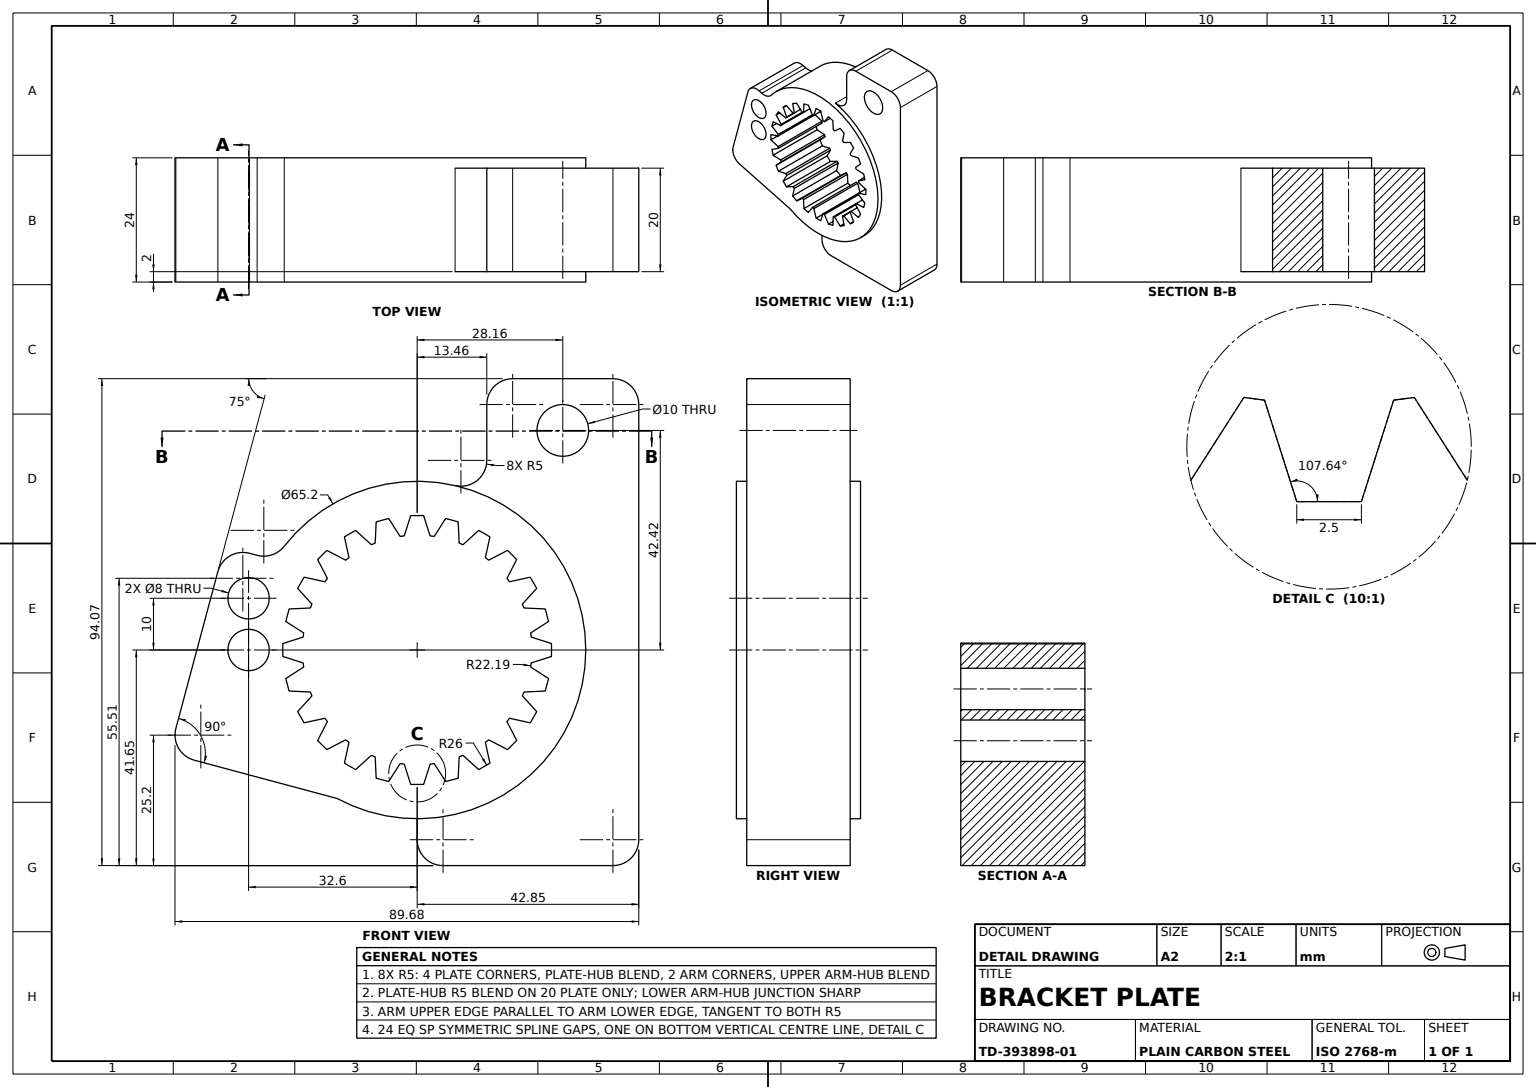
SolidWorks part; units mm, degrees
material "Plain Carbon Steel"
ref_plane "Front Plane" through (0, 0, 0) normal (0, 0, 1) x (1, 0, 0)
ref_plane "Top Plane" through (0, 0, 0) normal (0, 1, 0) x (1, 0, 0)
ref_plane "Right Plane" through (0, 0, 0) normal (1, 0, 0) x (0, 0, -1)
sketch "Splined Hub Profile" plane through (0, 0, 0) normal (0, 0, 1) x (1, 0, 0)
  line L0 (0, 0) -> (0, 32.6) construction
  line L1 (0, 0) -> (0, -32.6) construction
  line L2 (0, 0) -> (32.6, 0) construction
  line L3 (0, 0) -> (-32.6, 0) construction
  line L4 (26, 0) -> (25.97, 1.2496)
  line L5 (26, 0) -> (25.97, -1.2496)
  line L8 (22.0492, 2.496) -> (25.97, 1.2496)
  line L9 (22.0492, -2.496) -> (25.97, -1.2496)
  line L10 (21.9439, -3.2958) -> (25.4085, -5.5145)
  line L11 (20.6518, -8.1177) -> (24.7616, -7.9286)
  line L12 (20.3432, -8.863) -> (23.1155, -11.9028)
  line L13 (17.8471, -13.1862) -> (21.8658, -14.0672)
  line L14 (17.3561, -13.8262) -> (19.2472, -17.4799)
  line L15 (13.8262, -17.3561) -> (17.4799, -19.2472)
  line L16 (13.1862, -17.8471) -> (14.0672, -21.8658)
  line L17 (8.863, -20.3432) -> (11.9028, -23.1155)
  line L18 (8.1177, -20.6518) -> (7.9286, -24.7616)
  line L19 (3.2958, -21.9439) -> (5.5145, -25.4085)
  line L20 (2.496, -22.0492) -> (1.2496, -25.97)
  line L21 (-2.496, -22.0492) -> (-1.2496, -25.97)
  line L22 (-3.2958, -21.9439) -> (-5.5145, -25.4085)
  line L23 (-8.1177, -20.6518) -> (-7.9286, -24.7616)
  line L24 (-8.863, -20.3432) -> (-11.9028, -23.1155)
  line L25 (-13.1862, -17.8471) -> (-14.0672, -21.8658)
  line L26 (-13.8262, -17.3561) -> (-17.4799, -19.2472)
  line L27 (-17.3561, -13.8262) -> (-19.2472, -17.4799)
  line L28 (-17.8471, -13.1862) -> (-21.8658, -14.0672)
  line L29 (-20.3432, -8.863) -> (-23.1155, -11.9028)
  line L30 (-20.6518, -8.1177) -> (-24.7616, -7.9286)
  line L31 (-21.9439, -3.2958) -> (-25.4085, -5.5145)
  line L32 (-22.0492, -2.496) -> (-25.97, -1.2496)
  line L33 (-22.0492, 2.496) -> (-25.97, 1.2496)
  line L34 (-21.9439, 3.2958) -> (-25.4085, 5.5145)
  line L35 (-20.6518, 8.1177) -> (-24.7616, 7.9286)
  line L36 (-20.3432, 8.863) -> (-23.1155, 11.9028)
  line L37 (-17.8471, 13.1862) -> (-21.8658, 14.0672)
  line L38 (-17.3561, 13.8262) -> (-19.2472, 17.4799)
  line L39 (-13.8262, 17.3561) -> (-17.4799, 19.2472)
  line L40 (-13.1862, 17.8471) -> (-14.0672, 21.8658)
  line L41 (-8.863, 20.3432) -> (-11.9028, 23.1155)
  line L42 (-8.1177, 20.6518) -> (-7.9286, 24.7616)
  line L43 (-3.2958, 21.9439) -> (-5.5145, 25.4085)
  line L44 (-2.496, 22.0492) -> (-1.2496, 25.97)
  line L45 (2.496, 22.0492) -> (1.2496, 25.97)
  line L46 (3.2958, 21.9439) -> (5.5145, 25.4085)
  line L47 (8.1177, 20.6518) -> (7.9286, 24.7616)
  line L48 (8.863, 20.3432) -> (11.9028, 23.1155)
  line L49 (13.1862, 17.8471) -> (14.0672, 21.8658)
  line L50 (13.8262, 17.3561) -> (17.4799, 19.2472)
  line L51 (17.3561, 13.8262) -> (19.2472, 17.4799)
  line L52 (17.8471, 13.1862) -> (21.8658, 14.0672)
  line L53 (20.3432, 8.863) -> (23.1155, 11.9028)
  line L54 (20.6518, 8.1177) -> (24.7616, 7.9286)
  line L55 (21.9439, 3.2958) -> (25.4085, 5.5145)
  circle A0 centre (0, 0) radius 32.6
  arc A1 (25.4085, 5.5145) -> (24.7616, 7.9286) centre (0, 0) ccw
  arc A2 (3.2958, 21.9439) -> (2.496, 22.0492) centre (0, 0) ccw
  arc A3 (23.1155, 11.9028) -> (21.8658, 14.0672) centre (0, 0) ccw
  arc A4 (19.2472, 17.4799) -> (17.4799, 19.2472) centre (0, 0) ccw
  arc A5 (14.0672, 21.8658) -> (11.9028, 23.1155) centre (0, 0) ccw
  arc A6 (7.9286, 24.7616) -> (5.5145, 25.4085) centre (0, 0) ccw
  arc A7 (1.2496, 25.97) -> (-1.2496, 25.97) centre (0, 0) ccw
  arc A8 (-5.5145, 25.4085) -> (-7.9286, 24.7616) centre (0, 0) ccw
  arc A9 (-11.9028, 23.1155) -> (-14.0672, 21.8658) centre (0, 0) ccw
  arc A10 (-17.4799, 19.2472) -> (-19.2472, 17.4799) centre (0, 0) ccw
  arc A11 (-21.8658, 14.0672) -> (-23.1155, 11.9028) centre (0, 0) ccw
  arc A12 (-24.7616, 7.9286) -> (-25.4085, 5.5145) centre (0, 0) ccw
  arc A13 (-25.97, 1.2496) -> (-25.97, -1.2496) centre (0, 0) ccw
  arc A14 (-25.4085, -5.5145) -> (-24.7616, -7.9286) centre (0, 0) ccw
  arc A15 (-23.1155, -11.9028) -> (-21.8658, -14.0672) centre (0, 0) ccw
  arc A16 (-19.2472, -17.4799) -> (-17.4799, -19.2472) centre (0, 0) ccw
  arc A17 (-14.0672, -21.8658) -> (-11.9028, -23.1155) centre (0, 0) ccw
  arc A18 (-7.9286, -24.7616) -> (-5.5145, -25.4085) centre (0, 0) ccw
  arc A19 (-1.2496, -25.97) -> (1.2496, -25.97) centre (0, 0) ccw
  arc A20 (5.5145, -25.4085) -> (7.9286, -24.7616) centre (0, 0) ccw
  arc A21 (11.9028, -23.1155) -> (14.0672, -21.8658) centre (0, 0) ccw
  arc A22 (17.4799, -19.2472) -> (19.2472, -17.4799) centre (0, 0) ccw
  arc A23 (21.8658, -14.0672) -> (23.1155, -11.9028) centre (0, 0) ccw
  arc A24 (24.7616, -7.9286) -> (25.4085, -5.5145) centre (0, 0) ccw
  arc A25 (25.97, -1.2496) -> (25.97, 1.2496) centre (0, 0) ccw
  arc A26 (-2.496, 22.0492) -> (-3.2958, 21.9439) centre (0, 0) ccw
  arc A27 (-8.1177, 20.6518) -> (-8.863, 20.3432) centre (0, 0) ccw
  arc A28 (-13.1862, 17.8471) -> (-13.8262, 17.3561) centre (0, 0) ccw
  arc A29 (-17.3561, 13.8262) -> (-17.8471, 13.1862) centre (0, 0) ccw
  arc A30 (-20.3432, 8.863) -> (-20.6518, 8.1177) centre (0, 0) ccw
  arc A31 (-21.9439, 3.2958) -> (-22.0492, 2.496) centre (0, 0) ccw
  arc A32 (-22.0492, -2.496) -> (-21.9439, -3.2958) centre (0, 0) ccw
  arc A33 (-20.6518, -8.1177) -> (-20.3432, -8.863) centre (0, 0) ccw
  arc A34 (-17.8471, -13.1862) -> (-17.3561, -13.8262) centre (0, 0) ccw
  arc A35 (-13.8262, -17.3561) -> (-13.1862, -17.8471) centre (0, 0) ccw
  arc A36 (-8.863, -20.3432) -> (-8.1177, -20.6518) centre (0, 0) ccw
  arc A37 (-3.2958, -21.9439) -> (-2.496, -22.0492) centre (0, 0) ccw
  arc A38 (2.496, -22.0492) -> (3.2958, -21.9439) centre (0, 0) ccw
  arc A39 (8.1177, -20.6518) -> (8.863, -20.3432) centre (0, 0) ccw
  arc A40 (13.1862, -17.8471) -> (13.8262, -17.3561) centre (0, 0) ccw
  arc A41 (17.3561, -13.8262) -> (17.8471, -13.1862) centre (0, 0) ccw
  arc A42 (20.3432, -8.863) -> (20.6518, -8.1177) centre (0, 0) ccw
  arc A43 (21.9439, -3.2958) -> (21.9439, 3.2958) centre (0, 0) ccw
  arc A44 (20.6518, 8.1177) -> (20.3432, 8.863) centre (0, 0) ccw
  arc A45 (17.8471, 13.1862) -> (17.3561, 13.8262) centre (0, 0) ccw
  arc A46 (13.8262, 17.3561) -> (13.1862, 17.8471) centre (0, 0) ccw
  arc A47 (8.863, 20.3432) -> (8.1177, 20.6518) centre (0, 0) ccw
  dimension "D1" = 65.2
  dimension "D4" = 24
  dimension "D5" = 3.2958
  dimension "D6" = 5.5145
  dimension "D7" = 3.4646
  dimension "D8" = 3.9208
  dimension "D9" = 1.2496
  dimension "D10" = 5.5145
extrude "Splined Hub 24T" add sketch "Splined Hub Profile" along normal mid plane 24 contours A0 A47 L48 A5 L49 A46 L50 A4 L51 A45 L52 A3 L53 A44 L54 A1 L55 A43 L8 A25 L9 L10 A24 L11 A42 L12 A23 L13 A41 L14 A22 L15 A40 L16 A21 L17 A39 L18 A20 L19 A38 L20 A19 L21 A37 L22 A18 L23
ref_plane "Plane1" through (0, 0, 0) normal (0, 0, 1) x (1, 0, 0)
sketch "Mounting Flange Profile" plane through (0, 0, 0) normal (0, 0, 1) x (1, 0, 0)
  line L1 (42.85, 0) -> (42.85, -36.65)
  line L2 (37.85, -41.65) -> (5, -41.65)
  line L3 (0, -36.65) -> (0, -32.6)
  line L4 (42.85, 47.42) -> (42.85, 0)
  line L5 (37.85, 52.42) -> (18.46, 52.42)
  line L6 (13.46, 47.42) -> (13.46, 36.6359)
  arc A1 (13.46, 47.42) -> (18.46, 52.42) centre (18.46, 47.42) cw
  arc A2 (37.85, 52.42) -> (42.85, 47.42) centre (37.85, 47.42) cw
  arc A3 (42.85, -36.65) -> (37.85, -41.65) centre (37.85, -36.65) cw
  arc A4 (5, -41.65) -> (0, -36.65) centre (5, -36.65) cw
  arc A5 (7.335, 31.7641) -> (13.46, 36.6359) centre (8.46, 36.6359) ccw
  arc A6 (0, -32.6) -> (7.335, 31.7641) centre (0, 0) ccw
  point P12 (13.46, 52.42)
  point P15 (42.85, 52.42)
  dimension "D4" = 5
  dimension "D5" = 36.65
  dimension "D6" = 65.2
  dimension "D7" = 5
  dimension "D1" = 29.39
  dimension "D2" = 47.42
  dimension "D3" = 42.85
  dimension "D8" = 41.65
extrude "Mounting Flange" add sketch "Mounting Flange Profile" along normal mid plane 20
sketch "Side Lug Profile" plane through (0, 0, 0) normal (0, 0, 1) x (1, 0, 0)
  line L1 (-32.6, 0) -> (-42.6, 0) construction
  line L5 (-37.2463, 19.9802) -> (-47.955, -19.985)
  line L7 (-37.2463, 19.9802) -> (-27.5752, 17.3888)
  line L8 (-47.955, -19.985) -> (-15.4932, -28.6831)
  circle A0 centre (0, 0) radius 32.6 construction
  arc A1 (-27.5752, 17.3888) -> (-15.4932, -28.6831) centre (0, 0) ccw
  dimension "D6" = 65.2
  dimension "D7" = 15.4932
  dimension "D1" = 10
  dimension "D2" = 37.2463
  dimension "D3" = 17.3888
  dimension "D4" = 20.685
  dimension "D5" = 20.69
extrude "Side Lug" add sketch "Side Lug Profile" along normal mid plane 24
sketch "Lug Hole Profile" plane through (0, 0, 0) normal (0, 0, 1) x (1, 0, 0)
  circle A0 centre (28.155, 42.42) radius 5
  dimension "D1" = 10
  dimension "D2" = 42.42
  dimension "D3" = 28.155
extrude "Lug Hole Ø10" cut sketch "Lug Hole Profile" against normal mid plane 20
fillet "Lug Fillet R5" radius 5 3 edges at (-47.955, -19.985, 0) (-27.5752, 17.3888, 0) (-37.2463, 19.9802, 0)
sketch "Flange Holes Profile" plane through (0, 0, 10) normal (0, 0, 1) x (1, 0, 0)
  line L0 (42.85, 0) -> (-32.6, 0) construction
  line L1 (42.85, -36.65) -> (42.85, 47.42) construction
  circle A0 centre (-32.6, 0) radius 4
  dimension "D1" = 8
  dimension "D2" = 32.6
extrude "Flange Holes 2xØ8" cut sketch "Flange Holes Profile" against normal through all
ref_plane "Plane2" through (0, 0, 0) normal (0, 0, 1) x (1, 0, 0)
sketch "Flange Slot Profile" plane through (0, 0, 0) normal (0, 0, 1) x (1, 0, 0)
  line L0 (37.85, -41.65) -> (42.85, -41.65) construction
  line L3 (5, -41.65) -> (37.85, -41.65) construction
  line L4 (42.85, -41.65) -> (42.85, 0) construction
  line L5 (42.85, -36.65) -> (42.85, 47.42) construction
  line L6 (42.85, 0) -> (-32.6, 0) construction
  line L7 (-32.6, 0) -> (-32.6, 10) construction
  circle A0 centre (-32.6, 0) radius 4
  circle A1 centre (-32.6, 10) radius 4
  dimension "D1" = 8
  dimension "D3" = 8
  dimension "D2" = 32.6
  dimension "D4" = 10
extrude "Flange Slot" cut sketch "Flange Slot Profile" against normal mid plane 24
